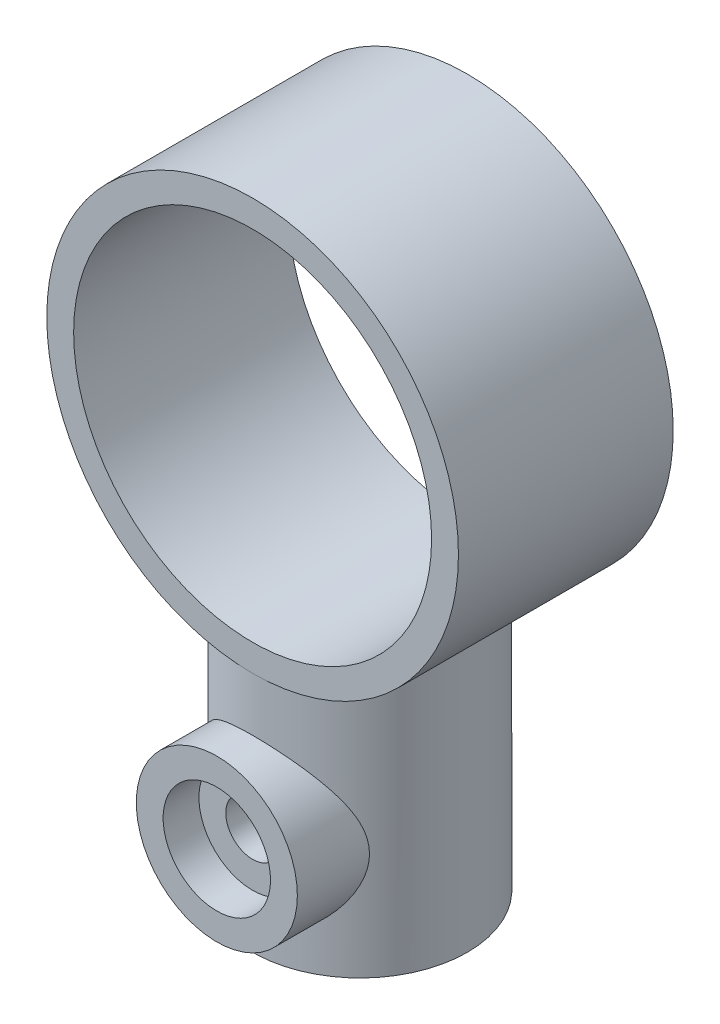
ISO-10303-21;
HEADER;
FILE_DESCRIPTION(('STEP AP214'),'2;1');
FILE_NAME('part.step','',(''),(''),'','','');
FILE_SCHEMA(('AUTOMOTIVE_DESIGN { 1 0 10303 214 1 1 1 1 }'));
ENDSEC;
DATA;
#1=APPLICATION_CONTEXT('core data for automotive mechanical design processes');
#2=APPLICATION_PROTOCOL_DEFINITION('international standard','automotive_design',2000,#1);
#3=PRODUCT_CONTEXT('',#1,'mechanical');
#4=PRODUCT('Part','Part','',(#3));
#5=PRODUCT_RELATED_PRODUCT_CATEGORY('part','',(#4));
#6=PRODUCT_DEFINITION_FORMATION('','',#4);
#7=PRODUCT_DEFINITION_CONTEXT('part definition',#1,'design');
#8=PRODUCT_DEFINITION('design','',#6,#7);
#9=PRODUCT_DEFINITION_SHAPE('','',#8);
#10=(LENGTH_UNIT() NAMED_UNIT(*) SI_UNIT(.MILLI.,.METRE.));
#11=(NAMED_UNIT(*) PLANE_ANGLE_UNIT() SI_UNIT($,.RADIAN.));
#12=(NAMED_UNIT(*) SI_UNIT($,.STERADIAN.) SOLID_ANGLE_UNIT());
#13=UNCERTAINTY_MEASURE_WITH_UNIT(LENGTH_MEASURE(1.E-05),#10,'distance_accuracy_value','');
#14=(GEOMETRIC_REPRESENTATION_CONTEXT(3) GLOBAL_UNCERTAINTY_ASSIGNED_CONTEXT((#13)) GLOBAL_UNIT_ASSIGNED_CONTEXT((#10,
#11,#12)) REPRESENTATION_CONTEXT('',''));
#15=CARTESIAN_POINT('',(0.,0.,0.));
#16=DIRECTION('',(0.,0.,1.));
#17=DIRECTION('',(1.,0.,0.));
#18=AXIS2_PLACEMENT_3D('',#15,#16,#17);
#19=CARTESIAN_POINT('',(0.,-19.,2.));
#20=DIRECTION('',(0.,0.,1.));
#21=DIRECTION('',(1.,0.,0.));
#22=AXIS2_PLACEMENT_3D('',#19,#20,#21);
#23=CYLINDRICAL_SURFACE('',#22,1.5);
#24=CARTESIAN_POINT('',(0.,-19.,6.));
#25=DIRECTION('',(0.,0.,1.));
#26=DIRECTION('',(1.,0.,0.));
#27=AXIS2_PLACEMENT_3D('',#24,#25,#26);
#28=CIRCLE('',#27,1.5);
#29=CARTESIAN_POINT('',(1.5,-19.,6.));
#30=VERTEX_POINT('',#29);
#31=EDGE_CURVE('E110',#30,#30,#28,.T.);
#32=ORIENTED_EDGE('',*,*,#31,.T.);
#33=EDGE_LOOP('',(#32));
#34=FACE_BOUND('',#33,.T.);
#35=CARTESIAN_POINT('',(0.,-19.,3.70809924354776));
#36=DIRECTION('',(0.,0.,-1.));
#37=DIRECTION('',(0.,1.,0.));
#38=AXIS2_PLACEMENT_3D('',#35,#36,#37);
#39=CIRCLE('',#38,1.5);
#40=CARTESIAN_POINT('',(-1.50000000000004,-18.9999999999999,3.70809924354776));
#41=VERTEX_POINT('',#40);
#42=CARTESIAN_POINT('',(1.49999999999977,-19.,3.70809924354776));
#43=VERTEX_POINT('',#42);
#44=EDGE_CURVE('E96',#41,#43,#39,.F.);
#45=ORIENTED_EDGE('',*,*,#44,.F.);
#46=EDGE_CURVE('E101',#43,#41,#39,.F.);
#47=ORIENTED_EDGE('',*,*,#46,.F.);
#48=EDGE_LOOP('',(#45,#47));
#49=FACE_BOUND('',#48,.T.);
#50=ADVANCED_FACE('F41',(#34,#49),#23,.F.);
#51=CARTESIAN_POINT('',(0.,-7.,3.70809924354776));
#52=DIRECTION('',(0.,0.,1.));
#53=DIRECTION('',(1.,0.,0.));
#54=AXIS2_PLACEMENT_3D('',#51,#52,#53);
#55=PLANE('',#54);
#56=ORIENTED_EDGE('',*,*,#46,.T.);
#57=DIRECTION('',(0.,-1.,0.));
#58=VECTOR('',#57,1.);
#59=CARTESIAN_POINT('',(-1.49999999999987,-6.99999999999999,3.70809924354776));
#60=LINE('',#59,#58);
#61=CARTESIAN_POINT('',(-1.49999999999991,-11.4017542509914,3.70809924354776));
#62=VERTEX_POINT('',#61);
#63=EDGE_CURVE('E83',#62,#41,#60,.T.);
#64=ORIENTED_EDGE('',*,*,#63,.F.);
#65=CARTESIAN_POINT('',(0.,0.,3.70809924354776));
#66=DIRECTION('',(0.,0.,1.));
#67=DIRECTION('',(1.,0.,0.));
#68=AXIS2_PLACEMENT_3D('',#65,#66,#67);
#69=CIRCLE('',#68,11.5);
#70=CARTESIAN_POINT('',(1.5000000000001,-11.4017542509914,3.70809924354776));
#71=VERTEX_POINT('',#70);
#72=EDGE_CURVE('E63',#62,#71,#69,.T.);
#73=ORIENTED_EDGE('',*,*,#72,.T.);
#74=DIRECTION('',(0.,-1.,0.));
#75=VECTOR('',#74,1.);
#76=CARTESIAN_POINT('',(1.50000000000013,-7.00000000000001,3.70809924354776));
#77=LINE('',#76,#75);
#78=EDGE_CURVE('E56',#71,#43,#77,.T.);
#79=ORIENTED_EDGE('',*,*,#78,.T.);
#80=EDGE_LOOP('',(#56,#64,#73,#79));
#81=FACE_BOUND('',#80,.T.);
#82=ADVANCED_FACE('F104',(#81),#55,.F.);
#83=CARTESIAN_POINT('',(0.,0.,6.));
#84=DIRECTION('',(0.,0.,1.));
#85=DIRECTION('',(1.,0.,0.));
#86=AXIS2_PLACEMENT_3D('',#83,#84,#85);
#87=PLANE('',#86);
#88=CARTESIAN_POINT('',(0.,0.,6.));
#89=DIRECTION('',(0.,0.,1.));
#90=DIRECTION('',(1.,0.,0.));
#91=AXIS2_PLACEMENT_3D('',#88,#89,#90);
#92=CIRCLE('',#91,11.5);
#93=CARTESIAN_POINT('',(0.,-11.5,6.));
#94=VERTEX_POINT('',#93);
#95=EDGE_CURVE('E51',#94,#94,#92,.T.);
#96=ORIENTED_EDGE('',*,*,#95,.T.);
#97=EDGE_LOOP('',(#96));
#98=FACE_BOUND('',#97,.T.);
#99=CARTESIAN_POINT('',(0.,0.,6.));
#100=DIRECTION('',(0.,0.,1.));
#101=DIRECTION('',(1.,0.,0.));
#102=AXIS2_PLACEMENT_3D('',#99,#100,#101);
#103=CIRCLE('',#102,10.);
#104=CARTESIAN_POINT('',(10.,0.,6.));
#105=VERTEX_POINT('',#104);
#106=EDGE_CURVE('E163',#105,#105,#103,.T.);
#107=ORIENTED_EDGE('',*,*,#106,.F.);
#108=EDGE_LOOP('',(#107));
#109=FACE_BOUND('',#108,.T.);
#110=ADVANCED_FACE('F180',(#98,#109),#87,.T.);
#111=CARTESIAN_POINT('',(0.,0.,-6.));
#112=DIRECTION('',(0.,0.,1.));
#113=DIRECTION('',(1.,0.,0.));
#114=AXIS2_PLACEMENT_3D('',#111,#112,#113);
#115=PLANE('',#114);
#116=CARTESIAN_POINT('',(0.,0.,-6.));
#117=DIRECTION('',(0.,0.,1.));
#118=DIRECTION('',(1.,0.,0.));
#119=AXIS2_PLACEMENT_3D('',#116,#117,#118);
#120=CIRCLE('',#119,11.5);
#121=CARTESIAN_POINT('',(0.,-11.5,-6.));
#122=VERTEX_POINT('',#121);
#123=EDGE_CURVE('E46',#122,#122,#120,.T.);
#124=ORIENTED_EDGE('',*,*,#123,.F.);
#125=EDGE_LOOP('',(#124));
#126=FACE_BOUND('',#125,.T.);
#127=CARTESIAN_POINT('',(0.,0.,-6.));
#128=DIRECTION('',(0.,0.,1.));
#129=DIRECTION('',(1.,0.,0.));
#130=AXIS2_PLACEMENT_3D('',#127,#128,#129);
#131=CIRCLE('',#130,10.);
#132=CARTESIAN_POINT('',(10.,0.,-6.));
#133=VERTEX_POINT('',#132);
#134=EDGE_CURVE('E152',#133,#133,#131,.T.);
#135=ORIENTED_EDGE('',*,*,#134,.T.);
#136=EDGE_LOOP('',(#135));
#137=FACE_BOUND('',#136,.T.);
#138=ADVANCED_FACE('F172',(#126,#137),#115,.F.);
#139=CARTESIAN_POINT('',(0.,0.,6.));
#140=DIRECTION('',(0.,0.,-1.));
#141=DIRECTION('',(-1.,0.,0.));
#142=AXIS2_PLACEMENT_3D('',#139,#140,#141);
#143=CYLINDRICAL_SURFACE('',#142,11.5);
#144=ORIENTED_EDGE('',*,*,#95,.F.);
#145=CARTESIAN_POINT('',(0.,-11.5,6.));
#146=CARTESIAN_POINT('',(0.156949578827933,-11.5000001355779,6.00000018262044));
#147=CARTESIAN_POINT('',(0.313897541694739,-11.496779962264,5.99383515190377));
#148=CARTESIAN_POINT('',(0.6266267232127,-11.4839818639018,5.969250324293));
#149=CARTESIAN_POINT('',(0.78240748044368,-11.4744015461444,5.95082591537107));
#150=CARTESIAN_POINT('',(1.09175175440838,-11.4491131770511,5.90191753135049));
#151=CARTESIAN_POINT('',(1.24531231034325,-11.4333976079975,5.87141876050534));
#152=CARTESIAN_POINT('',(1.54898348882044,-11.3962303126682,5.79871024455503));
#153=CARTESIAN_POINT('',(1.69909267420183,-11.374776242212,5.75649571329124));
#154=CARTESIAN_POINT('',(1.99416223199399,-11.3267626640489,5.66102891920833));
#155=CARTESIAN_POINT('',(2.13914255885142,-11.3002263208967,5.60782665445636));
#156=CARTESIAN_POINT('',(2.42383122801691,-11.242605583116,5.49078903598036));
#157=CARTESIAN_POINT('',(2.56353755744212,-11.2115194736562,5.42694967181545));
#158=CARTESIAN_POINT('',(2.97347192891126,-11.1124815994392,5.22033899187204));
#159=CARTESIAN_POINT('',(3.23482328089995,-11.0386979829443,5.06237435139018));
#160=CARTESIAN_POINT('',(3.74452958045316,-10.8767973262684,4.69923611516626));
#161=CARTESIAN_POINT('',(3.99097418237572,-10.7880643171826,4.49168348355608));
#162=CARTESIAN_POINT('',(4.44746391289357,-10.6080279075606,4.04018397814692));
#163=CARTESIAN_POINT('',(4.6574786381418,-10.5167224332789,3.79620701855532));
#164=CARTESIAN_POINT('',(4.95003726679143,-10.3807564849467,3.39525217625011));
#165=CARTESIAN_POINT('',(5.0470245263247,-10.3338194266377,3.24936331256475));
#166=CARTESIAN_POINT('',(5.22825678412554,-10.243318226809,2.94891015824408));
#167=CARTESIAN_POINT('',(5.31250719341773,-10.1997526568336,2.79434959010944));
#168=CARTESIAN_POINT('',(5.46751898205408,-10.1175068939615,2.47737077950324));
#169=CARTESIAN_POINT('',(5.53828138782099,-10.0788263293966,2.31495313612708));
#170=CARTESIAN_POINT('',(5.66549605291689,-10.007870040671,1.98334549078617));
#171=CARTESIAN_POINT('',(5.72195711983356,-9.97559037714009,1.81415973172985));
#172=CARTESIAN_POINT('',(5.81683662761796,-9.92054619063598,1.48073913098547));
#173=CARTESIAN_POINT('',(5.85614780407474,-9.8973202433967,1.3168349660179));
#174=CARTESIAN_POINT('',(5.92092061333041,-9.85870819120579,0.985481152489067));
#175=CARTESIAN_POINT('',(5.94638992234954,-9.84331774125878,0.818033522652497));
#176=CARTESIAN_POINT('',(5.98307546018686,-9.82106263754181,0.481141485903813));
#177=CARTESIAN_POINT('',(5.99430220671722,-9.81419169245379,0.311698645834845));
#178=CARTESIAN_POINT('',(6.00233545828585,-9.80928110826301,-0.0276480579803441));
#179=CARTESIAN_POINT('',(5.99914357072096,-9.81124048475133,-0.197551868226959));
#180=CARTESIAN_POINT('',(5.97979128876463,-9.82304398186212,-0.513523609621449));
#181=CARTESIAN_POINT('',(5.96541862727505,-9.83180084202554,-0.659746262263788));
#182=CARTESIAN_POINT('',(5.92608183096432,-9.85556101429158,-0.950290027245844));
#183=CARTESIAN_POINT('',(5.90111441248928,-9.87056626294257,-1.09461053574011));
#184=CARTESIAN_POINT('',(5.84088654816266,-9.90632463124338,-1.38034672465066));
#185=CARTESIAN_POINT('',(5.80562691028421,-9.92707729969527,-1.52176263215529));
#186=CARTESIAN_POINT('',(5.72519555337451,-9.97367980424175,-1.80090697735693));
#187=CARTESIAN_POINT('',(5.68001991596391,-9.99953165490475,-1.93863393312992));
#188=CARTESIAN_POINT('',(5.52798396598323,-10.0848968911938,-2.35127008986333));
#189=CARTESIAN_POINT('',(5.40595529204071,-10.1513811071149,-2.61932137568859));
#190=CARTESIAN_POINT('',(5.12582570187856,-10.2956624209485,-3.13233832170076));
#191=CARTESIAN_POINT('',(4.96770863914086,-10.3734645770196,-3.37729357882386));
#192=CARTESIAN_POINT('',(4.59418299191631,-10.5447319025564,-3.87335238223689));
#193=CARTESIAN_POINT('',(4.37385657367147,-10.6388667848999,-4.12053410943194));
#194=CARTESIAN_POINT('',(3.8945238655214,-10.8235162312259,-4.5762402813956));
#195=CARTESIAN_POINT('',(3.63549598915194,-10.9140287388105,-4.78474300580679));
#196=CARTESIAN_POINT('',(3.2143211161667,-11.0427084943076,-5.06942258731698));
#197=CARTESIAN_POINT('',(3.06415302608544,-11.0854180973587,-5.16160643824063));
#198=CARTESIAN_POINT('',(2.75534105655058,-11.1661770963876,-5.33284393580427));
#199=CARTESIAN_POINT('',(2.59670081324246,-11.2042284688993,-5.41190315646262));
#200=CARTESIAN_POINT('',(2.27203832366371,-11.274547726851,-5.55602186298455));
#201=CARTESIAN_POINT('',(2.10601941978374,-11.3068181982645,-5.62108761118107));
#202=CARTESIAN_POINT('',(1.76778722899716,-11.3646092392143,-5.73644830342684));
#203=CARTESIAN_POINT('',(1.59557472936085,-11.3901306632039,-5.78674511736463));
#204=CARTESIAN_POINT('',(1.26171558673617,-11.4317037739775,-5.86813103172292));
#205=CARTESIAN_POINT('',(1.10046276945584,-11.4483886224873,-5.90051563500229));
#206=CARTESIAN_POINT('',(0.775301200908844,-11.4749948435218,-5.9519739570192));
#207=CARTESIAN_POINT('',(0.611392714773712,-11.4849168870103,-5.9710489962542));
#208=CARTESIAN_POINT('',(0.282358074725133,-11.4977115427036,-5.99562178270494));
#209=CARTESIAN_POINT('',(0.117232478147314,-11.5005872021086,-6.00112539887258));
#210=CARTESIAN_POINT('',(-0.212876139333233,-11.4992139337846,-5.99849344051178));
#211=CARTESIAN_POINT('',(-0.377859167245579,-11.494965378924,-5.99035857979601));
#212=CARTESIAN_POINT('',(-0.692077607348148,-11.4801392838329,-5.96185612461983));
#213=CARTESIAN_POINT('',(-0.841443338858839,-11.4701395533605,-5.94260475543453));
#214=CARTESIAN_POINT('',(-1.1378856895511,-11.4445338372521,-5.89303027605832));
#215=CARTESIAN_POINT('',(-1.28496157460343,-11.4289260907783,-5.8627036883562));
#216=CARTESIAN_POINT('',(-1.57576547001364,-11.3924726565118,-5.791318826621));
#217=CARTESIAN_POINT('',(-1.71949451694579,-11.3716286147179,-5.7502639248081));
#218=CARTESIAN_POINT('',(-2.00284565139837,-11.3251593447799,-5.65781144649547));
#219=CARTESIAN_POINT('',(-2.1424661144892,-11.2995322541789,-5.6064098405095));
#220=CARTESIAN_POINT('',(-2.42036025169921,-11.2433297744297,-5.49226711627424));
#221=CARTESIAN_POINT('',(-2.55850470284527,-11.212643127812,-5.42926609647112));
#222=CARTESIAN_POINT('',(-2.82894302130084,-11.1474867251274,-5.29339248396464));
#223=CARTESIAN_POINT('',(-2.96123488974975,-11.1130156903428,-5.22051655263843));
#224=CARTESIAN_POINT('',(-3.3483703143814,-11.0050011672394,-4.98788532913089));
#225=CARTESIAN_POINT('',(-3.59362293177143,-10.9268248816615,-4.81406476637323));
#226=CARTESIAN_POINT('',(-4.07845441766789,-10.7558845893354,-4.41308062583474));
#227=CARTESIAN_POINT('',(-4.31476155891889,-10.6624498887889,-4.18224068751647));
#228=CARTESIAN_POINT('',(-4.63865684293523,-10.5236283447289,-3.80920784754676));
#229=CARTESIAN_POINT('',(-4.74159614201426,-10.4775407642408,-3.68029020728233));
#230=CARTESIAN_POINT('',(-4.93679704899914,-10.3869914671592,-3.41398249926734));
#231=CARTESIAN_POINT('',(-5.02905693172337,-10.3425300140459,-3.2765910681174));
#232=CARTESIAN_POINT('',(-5.2075334781137,-10.2538835713497,-2.98538298472546));
#233=CARTESIAN_POINT('',(-5.29304089939074,-10.2098799999887,-2.83107557841413));
#234=CARTESIAN_POINT('',(-5.45053097521659,-10.126679772442,-2.51454537611282));
#235=CARTESIAN_POINT('',(-5.52252016002734,-10.0874807984915,-2.35232644990204));
#236=CARTESIAN_POINT('',(-5.65216403762056,-10.0154153379937,-2.02105131937275));
#237=CARTESIAN_POINT('',(-5.70983122240028,-9.98254333857718,-1.85200122409345));
#238=CARTESIAN_POINT('',(-5.81010867727679,-9.9245153269321,-1.5082048281158));
#239=CARTESIAN_POINT('',(-5.85272151536941,-9.89935799881859,-1.33345950447928));
#240=CARTESIAN_POINT('',(-5.91879845654428,-9.8599773571974,-0.997125596417495));
#241=CARTESIAN_POINT('',(-5.94372747316176,-9.84492546066,-0.835921212389537));
#242=CARTESIAN_POINT('',(-5.98038742493029,-9.82269981291726,-0.511477725647174));
#243=CARTESIAN_POINT('',(-5.99211929476964,-9.81552550378242,-0.348238767859585));
#244=CARTESIAN_POINT('',(-6.00219018121771,-9.8093704244503,-0.0212746956513013));
#245=CARTESIAN_POINT('',(-6.00053582448525,-9.81038560016566,0.142450138120795));
#246=CARTESIAN_POINT('',(-5.98387835527532,-9.82055469279135,0.468955429442394));
#247=CARTESIAN_POINT('',(-5.96887599193873,-9.82970815295021,0.63173593947489));
#248=CARTESIAN_POINT('',(-5.92819127728147,-9.85429043436735,0.936742751821818));
#249=CARTESIAN_POINT('',(-5.90389851592604,-9.86889848594337,1.07922324730548));
#250=CARTESIAN_POINT('',(-5.8452817746423,-9.90372810988931,1.36142472318204));
#251=CARTESIAN_POINT('',(-5.81095451103383,-9.92395151971452,1.5011447842494));
#252=CARTESIAN_POINT('',(-5.69344223441867,-9.9921474078394,1.91488554677635));
#253=CARTESIAN_POINT('',(-5.59570137647601,-10.0476618132275,2.18367293189669));
#254=CARTESIAN_POINT('',(-5.35717564237041,-10.1769405832222,2.71886242225505));
#255=CARTESIAN_POINT('',(-5.21397923406328,-10.2516663146062,2.98394079537057));
#256=CARTESIAN_POINT('',(-4.89110956605737,-10.4095819630624,3.48808983239893));
#257=CARTESIAN_POINT('',(-4.71141672357178,-10.4927764121656,3.72714642766466));
#258=CARTESIAN_POINT('',(-4.29183181980609,-10.6718711921826,4.2065242224796));
#259=CARTESIAN_POINT('',(-4.04707182811816,-10.7679568339543,4.4425706468183));
#260=CARTESIAN_POINT('',(-3.65148746580848,-10.9057916851509,4.76399275734891));
#261=CARTESIAN_POINT('',(-3.51475503645127,-10.9507237321279,4.86576586077563));
#262=CARTESIAN_POINT('',(-3.23243661986418,-11.0373504171677,5.05771159354309));
#263=CARTESIAN_POINT('',(-3.08685463531819,-11.0790464997227,5.14788941081377));
#264=CARTESIAN_POINT('',(-2.78486276212116,-11.158825320879,5.31743165196371));
#265=CARTESIAN_POINT('',(-2.62830336717781,-11.196827869194,5.39656770964361));
#266=CARTESIAN_POINT('',(-2.30786598455693,-11.2672374830238,5.54117575722826));
#267=CARTESIAN_POINT('',(-2.14399164949471,-11.2996473027075,5.60665447609682));
#268=CARTESIAN_POINT('',(-1.81040554038446,-11.3578623353638,5.72307380861668));
#269=CARTESIAN_POINT('',(-1.64070671649361,-11.3836812442014,5.77404459543316));
#270=CARTESIAN_POINT('',(-1.29664056140096,-11.4279822417378,5.86090237441121));
#271=CARTESIAN_POINT('',(-1.12227597512963,-11.4464685472303,5.89679803659391));
#272=CARTESIAN_POINT('',(-0.79028551012749,-11.4738827208415,5.94982642127283));
#273=CARTESIAN_POINT('',(-0.632992460182356,-11.483654127812,5.96861998891456));
#274=CARTESIAN_POINT('',(-0.31713240879539,-11.4967127694845,5.99370682209347));
#275=CARTESIAN_POINT('',(-0.158565379695124,-11.4999998630263,5.99999981549947));
#276=CARTESIAN_POINT('',(0.,-11.5,6.));
#277=B_SPLINE_CURVE_WITH_KNOTS('',3,(#145,#146,#147,#148,#149,#150,#151,#152,#153,#154,#155,
#156,#157,#158,#159,#160,#161,#162,#163,#164,#165,#166,#167,#168,#169,#170,#171,#172,#173,#174,
#175,#176,#177,#178,#179,#180,#181,#182,#183,#184,#185,#186,#187,#188,#189,#190,#191,#192,#193,
#194,#195,#196,#197,#198,#199,#200,#201,#202,#203,#204,#205,#206,#207,#208,#209,#210,#211,#212,
#213,#214,#215,#216,#217,#218,#219,#220,#221,#222,#223,#224,#225,#226,#227,#228,#229,#230,#231,
#232,#233,#234,#235,#236,#237,#238,#239,#240,#241,#242,#243,#244,#245,#246,#247,#248,#249,#250,
#251,#252,#253,#254,#255,#256,#257,#258,#259,#260,#261,#262,#263,#264,#265,#266,#267,#268,#269,
#270,#271,#272,#273,#274,#275,#276),.UNSPECIFIED.,.T.,.F.,(4,2,2,2,2,2,2,2,2,2,2,2,2,2,2,2,2,2,
2,2,2,2,2,2,2,2,2,2,2,2,2,2,2,2,2,2,2,2,2,2,2,2,2,2,2,2,2,2,2,2,2,2,2,2,2,2,2,2,2,2,2,2,2,2,2,
4),(0.,0.470692988347527,0.941563153500217,1.41301211091961,1.88465395034882,2.35419515677509,
2.82391379370479,3.76237773296836,4.76106646584416,5.76058470750014,6.30410876981105,
6.8474012727456,7.39065241517701,7.93356817434236,8.4432575664312,8.95266401326091,
9.46169405906647,9.97066735933802,10.4117092732762,10.8528879801556,11.2940320623631,
11.7353507807,12.6372965018234,13.5396465616096,14.5680573329443,15.597043875982,
16.140352845317,16.6834304782373,17.2262645659939,17.7690298960917,18.2643078023531,
18.7595365630343,19.2545511248155,19.749539779258,20.2018125668466,20.6542274859734,
21.1065003686736,21.5589497293685,22.0231534673376,22.4875145420254,23.4157482798121,
24.4409922351983,24.9544170464423,25.4679246823015,26.0126762775516,26.557164038545,
27.1011752028526,27.6450935239605,28.1358290947884,28.6265299070667,29.1169878198374,
29.6074182079819,30.0427373760832,30.4781991573565,31.3485636603898,32.2762679094131,
33.2044712553565,34.2592761503955,34.7875907669549,35.3156681778426,35.8534199346152,
36.3909061122234,36.92726613486,37.4633172617339,37.9388456973503,38.4143844848669),.UNSPECIFIED.);
#278=EDGE_CURVE('E154',#94,#122,#277,.T.);
#279=ORIENTED_EDGE('',*,*,#278,.T.);
#280=ORIENTED_EDGE('',*,*,#123,.T.);
#281=EDGE_CURVE('E159',#122,#94,#277,.T.);
#282=ORIENTED_EDGE('',*,*,#281,.T.);
#283=EDGE_LOOP('',(#144,#279,#280,#282));
#284=FACE_BOUND('',#283,.T.);
#285=ADVANCED_FACE('F43',(#284),#143,.T.);
#286=CARTESIAN_POINT('',(0.,0.,6.));
#287=DIRECTION('',(0.,0.,-1.));
#288=DIRECTION('',(-1.,0.,0.));
#289=AXIS2_PLACEMENT_3D('',#286,#287,#288);
#290=CYLINDRICAL_SURFACE('',#289,10.);
#291=ORIENTED_EDGE('',*,*,#106,.T.);
#292=EDGE_LOOP('',(#291));
#293=FACE_BOUND('',#292,.T.);
#294=ORIENTED_EDGE('',*,*,#134,.F.);
#295=EDGE_LOOP('',(#294));
#296=FACE_BOUND('',#295,.T.);
#297=ADVANCED_FACE('F150',(#293,#296),#290,.F.);
#298=CARTESIAN_POINT('',(0.,-7.,0.));
#299=DIRECTION('',(0.,-1.,0.));
#300=DIRECTION('',(1.,0.,0.));
#301=AXIS2_PLACEMENT_3D('',#298,#299,#300);
#302=CYLINDRICAL_SURFACE('',#301,3.99999999999993);
#303=CARTESIAN_POINT('',(1.5,-25.,3.70809924354776));
#304=VERTEX_POINT('',#303);
#305=EDGE_CURVE('E91',#43,#304,#77,.T.);
#306=ORIENTED_EDGE('',*,*,#305,.F.);
#307=ORIENTED_EDGE('',*,*,#78,.F.);
#308=CARTESIAN_POINT('',(3.99999999999986,-10.781929326424,0.));
#309=CARTESIAN_POINT('',(4.00000314657652,-10.7819266948872,-0.217255336232914));
#310=CARTESIAN_POINT('',(3.98224047792889,-10.7885674998856,-0.434488763758288));
#311=CARTESIAN_POINT('',(3.91192630301894,-10.8142594176625,-0.862481103339597));
#312=CARTESIAN_POINT('',(3.85937154330999,-10.8333116910484,-1.07323940797085));
#313=CARTESIAN_POINT('',(3.72157378861011,-10.8814129934875,-1.48200382376832));
#314=CARTESIAN_POINT('',(3.6363995247052,-10.9104409900308,-1.68003573245359));
#315=CARTESIAN_POINT('',(3.43601854263587,-10.9751913442759,-2.05906879865697));
#316=CARTESIAN_POINT('',(3.32080431721443,-11.0109153747487,-2.2400656835589));
#317=CARTESIAN_POINT('',(3.05835039537032,-11.0867408076852,-2.58761009149744));
#318=CARTESIAN_POINT('',(2.9100429040825,-11.1269581781588,-2.75332615882137));
#319=CARTESIAN_POINT('',(2.58788673420046,-11.2062630333278,-3.05810823348963));
#320=CARTESIAN_POINT('',(2.41403354000832,-11.2453503167978,-3.19716951915368));
#321=CARTESIAN_POINT('',(2.03956351041542,-11.3193455391787,-3.44854433058932));
#322=CARTESIAN_POINT('',(1.83832180830089,-11.3541013537127,-3.55997575292531));
#323=CARTESIAN_POINT('',(1.41853124269149,-11.4141420626472,-3.74706935634629));
#324=CARTESIAN_POINT('',(1.19998750897693,-11.4394297515533,-3.82274209329461));
#325=CARTESIAN_POINT('',(0.760522326117555,-11.4768629954855,-3.93331855030355));
#326=CARTESIAN_POINT('',(0.539999668884433,-11.4894671957487,-3.96964898787937));
#327=CARTESIAN_POINT('',(0.0956518560104309,-11.5017473691412,-4.0050577250022));
#328=CARTESIAN_POINT('',(-0.128172356803093,-11.5014269643494,-4.00414646141529));
#329=CARTESIAN_POINT('',(-0.562628738311855,-11.4881984836479,-3.96597785288426));
#330=CARTESIAN_POINT('',(-0.773416363456932,-11.4758279465457,-3.930272591008));
#331=CARTESIAN_POINT('',(-1.18579631370684,-11.4405741640333,-3.82611095336748));
#332=CARTESIAN_POINT('',(-1.38738800209992,-11.4176901919009,-3.7576523135711));
#333=CARTESIAN_POINT('',(-1.77891248704159,-11.3633227238448,-3.58908505835547));
#334=CARTESIAN_POINT('',(-1.96864770310442,-11.3317257016856,-3.4885556579473));
#335=CARTESIAN_POINT('',(-2.32899682093034,-11.2631907969005,-3.25905514608549));
#336=CARTESIAN_POINT('',(-2.49960506659063,-11.2262513418015,-3.13007565484153));
#337=CARTESIAN_POINT('',(-2.82606513386257,-11.1486745512438,-2.83962735433131));
#338=CARTESIAN_POINT('',(-2.98072147863608,-11.1079447015802,-2.67683757838325));
#339=CARTESIAN_POINT('',(-3.26094797642742,-11.0289376993801,-2.32731693730578));
#340=CARTESIAN_POINT('',(-3.38651277882249,-10.9906609989707,-2.1405816778313));
#341=CARTESIAN_POINT('',(-3.60684990992326,-10.920360971299,-1.74437541164528));
#342=CARTESIAN_POINT('',(-3.7010718200857,-10.8884530012696,-1.53457624721657));
#343=CARTESIAN_POINT('',(-3.8524271261761,-10.8358341813979,-1.10069484305685));
#344=CARTESIAN_POINT('',(-3.90957773937398,-10.8151181343644,-0.876619286987419));
#345=CARTESIAN_POINT('',(-3.98263925841823,-10.7884212419073,-0.432210719646963));
#346=CARTESIAN_POINT('',(-4.00041969811956,-10.7817730993558,-0.212225215469678));
#347=CARTESIAN_POINT('',(-3.99956545239841,-10.7820910624059,0.227639507886412));
#348=CARTESIAN_POINT('',(-3.98093815848701,-10.789054404599,0.447518739575677));
#349=CARTESIAN_POINT('',(-3.90948277571084,-10.8151411210005,0.872074491886128));
#350=CARTESIAN_POINT('',(-3.8580010540821,-10.8337852906148,1.07701030192532));
#351=CARTESIAN_POINT('',(-3.7239397943008,-10.8805918133589,1.4752774913194));
#352=CARTESIAN_POINT('',(-3.64135444260578,-10.9087559457527,1.66860669346018));
#353=CARTESIAN_POINT('',(-3.44426879415293,-10.9726048973001,2.04541993178731));
#354=CARTESIAN_POINT('',(-3.32878445230759,-11.0085116691766,2.2283506225589));
#355=CARTESIAN_POINT('',(-3.07027059544534,-11.0833894368424,2.57290905730878));
#356=CARTESIAN_POINT('',(-2.92723227768871,-11.1223614095187,2.73452996552629));
#357=CARTESIAN_POINT('',(-2.60865742371181,-11.2014821658468,3.04076690570169));
#358=CARTESIAN_POINT('',(-2.43179808769057,-11.2415834741986,3.18402336891874));
#359=CARTESIAN_POINT('',(-2.05556021379345,-11.3164220998505,3.43893786266677));
#360=CARTESIAN_POINT('',(-1.85618224045722,-11.3511595515703,3.55059668510105));
#361=CARTESIAN_POINT('',(-1.44132125531167,-11.4112320794752,3.73819420931193));
#362=CARTESIAN_POINT('',(-1.22593857393044,-11.436620625482,3.81433673175178));
#363=CARTESIAN_POINT('',(-0.784357241241908,-11.4753568277292,3.92896429388479));
#364=CARTESIAN_POINT('',(-0.558162920245526,-11.488709262854,3.96746427989474));
#365=CARTESIAN_POINT('',(-0.113762111596045,-11.501476627674,4.00427643177558));
#366=CARTESIAN_POINT('',(0.104265596272577,-11.5015658253351,4.00453280420546));
#367=CARTESIAN_POINT('',(0.537113760489189,-11.4894896642182,3.96971528088925));
#368=CARTESIAN_POINT('',(0.751934515174897,-11.4773254526561,3.93464469260193));
#369=CARTESIAN_POINT('',(1.1682689825417,-11.4423785548636,3.83148907745086));
#370=CARTESIAN_POINT('',(1.36995572166124,-11.4197972370693,3.76402918727062));
#371=CARTESIAN_POINT('',(1.75920776274612,-11.3663462696473,3.59860185717365));
#372=CARTESIAN_POINT('',(1.94677043880624,-11.3354750836387,3.50062876163337));
#373=CARTESIAN_POINT('',(2.31041493756695,-11.2671005300579,3.27258612737591));
#374=CARTESIAN_POINT('',(2.48576658696086,-11.2293859263638,3.14141652896516));
#375=CARTESIAN_POINT('',(2.8125947319369,-11.1520208071119,2.85252769438948));
#376=CARTESIAN_POINT('',(2.96406324330576,-11.1123696499352,2.6947996159213));
#377=CARTESIAN_POINT('',(3.24557817237721,-11.0335192560423,2.34905234319778));
#378=CARTESIAN_POINT('',(3.37440059236079,-10.9944153308317,2.16001130869306));
#379=CARTESIAN_POINT('',(3.59839984489605,-10.9231587605909,1.76172989505965));
#380=CARTESIAN_POINT('',(3.69358164349432,-10.8910050898327,1.55249250313871));
#381=CARTESIAN_POINT('',(3.8458069995994,-10.838183085146,1.12288270167076));
#382=CARTESIAN_POINT('',(3.90342389063485,-10.8173429457616,0.90273569256634));
#383=CARTESIAN_POINT('',(3.98051046462658,-10.7892203865282,0.455048945321354));
#384=CARTESIAN_POINT('',(3.99999670486609,-10.7819320822016,0.227512459529251));
#385=CARTESIAN_POINT('',(3.99999999999986,-10.781929326424,0.));
#386=B_SPLINE_CURVE_WITH_KNOTS('',3,(#308,#309,#310,#311,#312,#313,#314,#315,#316,#317,#318,
#319,#320,#321,#322,#323,#324,#325,#326,#327,#328,#329,#330,#331,#332,#333,#334,#335,#336,#337,
#338,#339,#340,#341,#342,#343,#344,#345,#346,#347,#348,#349,#350,#351,#352,#353,#354,#355,#356,
#357,#358,#359,#360,#361,#362,#363,#364,#365,#366,#367,#368,#369,#370,#371,#372,#373,#374,#375,
#376,#377,#378,#379,#380,#381,#382,#383,#384,#385),.UNSPECIFIED.,.T.,.F.,(4,2,2,2,2,2,2,2,2,2,2,
2,2,2,2,2,2,2,2,2,2,2,2,2,2,2,2,2,2,2,2,2,2,2,2,2,2,2,4),(0.,0.650921909801569,1.301904696625,
1.95152330718617,2.60130441915738,3.27625918225249,3.95133339788453,4.64578028679665,
5.34002204868048,6.00814477227088,6.67608025791707,7.31552343393114,7.95501081696127,
8.60325980697967,9.25169999011812,9.93319342368778,10.6148121006922,11.3078365129701,
12.0005388284013,12.6595705401675,13.3184684689778,13.9519613616294,14.5855727184921,
15.2405921689976,15.8958212283479,16.5858602431942,17.2758819626803,17.9618935348493,
18.6476326090358,19.298497953293,19.9493023664602,20.5880220121539,21.2268601150802,
21.8905428059991,22.5544469000047,23.2473366731027,23.9401241186769,24.6220737318841,
25.3037271597275),.UNSPECIFIED.);
#387=EDGE_CURVE('E94',#71,#62,#386,.T.);
#388=ORIENTED_EDGE('',*,*,#387,.T.);
#389=ORIENTED_EDGE('',*,*,#63,.T.);
#390=CARTESIAN_POINT('',(-1.5,-25.,3.70809924354776));
#391=VERTEX_POINT('',#390);
#392=EDGE_CURVE('E87',#41,#391,#60,.T.);
#393=ORIENTED_EDGE('',*,*,#392,.T.);
#394=CARTESIAN_POINT('',(-1.74574066942157E-13,-25.,0.));
#395=DIRECTION('',(0.,-1.,0.));
#396=DIRECTION('',(1.,0.,0.));
#397=AXIS2_PLACEMENT_3D('',#394,#395,#396);
#398=CIRCLE('',#397,3.99999999999993);
#399=EDGE_CURVE('E304',#391,#304,#398,.T.);
#400=ORIENTED_EDGE('',*,*,#399,.T.);
#401=EDGE_LOOP('',(#306,#307,#388,#389,#393,#400));
#402=FACE_BOUND('',#401,.T.);
#403=ADVANCED_FACE('F90',(#402),#302,.F.);
#404=CARTESIAN_POINT('',(0.,-7.,0.));
#405=DIRECTION('',(0.,-1.,0.));
#406=DIRECTION('',(1.,0.,0.));
#407=AXIS2_PLACEMENT_3D('',#404,#405,#406);
#408=CYLINDRICAL_SURFACE('',#407,6.);
#409=CARTESIAN_POINT('',(4.5,-19.,3.96862696659674));
#410=CARTESIAN_POINT('',(4.50000507834795,-18.8949418488794,3.96861686602141));
#411=CARTESIAN_POINT('',(4.49631419586517,-18.7899195297317,3.9728168514459));
#412=CARTESIAN_POINT('',(4.48167225616228,-18.5809864703694,3.98932854522559));
#413=CARTESIAN_POINT('',(4.47071877665906,-18.4770761127793,4.00164295996579));
#414=CARTESIAN_POINT('',(4.44180872189387,-18.2711836297107,4.03370728475386));
#415=CARTESIAN_POINT('',(4.42383673572161,-18.1692062688658,4.0534735539058));
#416=CARTESIAN_POINT('',(4.38129405910782,-17.9680882523386,4.09941990164114));
#417=CARTESIAN_POINT('',(4.35671931259617,-17.8689493819012,4.12560392177298));
#418=CARTESIAN_POINT('',(4.2745464375733,-17.5794046616541,4.21122557626126));
#419=CARTESIAN_POINT('',(4.20803426948237,-17.3937238166576,4.2782871478847));
#420=CARTESIAN_POINT('',(4.05390989402713,-17.0369234945698,4.42460194939479));
#421=CARTESIAN_POINT('',(3.96630023685819,-16.865802260941,4.50385370535392));
#422=CARTESIAN_POINT('',(3.75120672461474,-16.5036814358669,4.68531341730841));
#423=CARTESIAN_POINT('',(3.61921460613341,-16.3160250828106,4.78885287141302));
#424=CARTESIAN_POINT('',(3.32798047453307,-15.9623946729377,4.99564919290693));
#425=CARTESIAN_POINT('',(3.16869833241079,-15.7964531900511,5.09890541333791));
#426=CARTESIAN_POINT('',(2.89258319383621,-15.5500278679837,5.25807588714212));
#427=CARTESIAN_POINT('',(2.78403025278295,-15.4617866905745,5.31649921498468));
#428=CARTESIAN_POINT('',(2.55764383078975,-15.2948357833496,5.42903557769024));
#429=CARTESIAN_POINT('',(2.43980827260277,-15.2161281970001,5.48314764230636));
#430=CARTESIAN_POINT('',(2.19555612221116,-15.0693791398114,5.58542936763));
#431=CARTESIAN_POINT('',(2.06915634837481,-15.0013175852969,5.63361018010819));
#432=CARTESIAN_POINT('',(1.80839242601433,-14.8768220679997,5.72264868834265));
#433=CARTESIAN_POINT('',(1.67403253937859,-14.8203819542008,5.76351025654372));
#434=CARTESIAN_POINT('',(1.34369921738147,-14.7004313389689,5.85098111190473));
#435=CARTESIAN_POINT('',(1.14436283139104,-14.6429432828994,5.89347882975045));
#436=CARTESIAN_POINT('',(0.736633167118957,-14.5558150938569,5.95818156512857));
#437=CARTESIAN_POINT('',(0.528247922690005,-14.5261507664387,5.98040421262311));
#438=CARTESIAN_POINT('',(0.107601910306231,-14.4963387137746,6.00273790900922));
#439=CARTESIAN_POINT('',(-0.104667502038748,-14.4962676849033,6.00279150279406));
#440=CARTESIAN_POINT('',(-0.525950245750392,-14.5258527620655,5.98062709423097));
#441=CARTESIAN_POINT('',(-0.734962811689901,-14.5555157523132,5.95840393422351));
#442=CARTESIAN_POINT('',(-1.1366671291912,-14.6412434187138,5.894741109369));
#443=CARTESIAN_POINT('',(-1.32967268311153,-14.6963690509536,5.85398567140417));
#444=CARTESIAN_POINT('',(-1.70304157676307,-14.8299868547386,5.75646842129022));
#445=CARTESIAN_POINT('',(-1.88340214926541,-14.9084841213365,5.69970311910817));
#446=CARTESIAN_POINT('',(-2.24765072773045,-15.0955888678264,5.56683136038156));
#447=CARTESIAN_POINT('',(-2.42980614387423,-15.2065362960667,5.48929621311769));
#448=CARTESIAN_POINT('',(-2.77370176192021,-15.4502011056958,5.32382107964188));
#449=CARTESIAN_POINT('',(-2.9354243570541,-15.5829370386549,5.23587224475466));
#450=CARTESIAN_POINT('',(-3.26724612468181,-15.8956700493885,5.03681297456608));
#451=CARTESIAN_POINT('',(-3.43273478808483,-16.0798276340312,4.92454967628694));
#452=CARTESIAN_POINT('',(-3.7320262687465,-16.4735037469118,4.70177874821722));
#453=CARTESIAN_POINT('',(-3.86581399076325,-16.683034285684,4.59127197811539));
#454=CARTESIAN_POINT('',(-4.07619618880002,-17.0829456210872,4.40458278221533));
#455=CARTESIAN_POINT('',(-4.15886599457748,-17.2689611706744,4.32592800158741));
#456=CARTESIAN_POINT('',(-4.299581924703,-17.6561958095648,4.1861022298521));
#457=CARTESIAN_POINT('',(-4.35768369642175,-17.8573793107592,4.12489183040217));
#458=CARTESIAN_POINT('',(-4.43707152670479,-18.231060934876,4.03920154203046));
#459=CARTESIAN_POINT('',(-4.46337197039467,-18.4013415947896,4.00984626605542));
#460=CARTESIAN_POINT('',(-4.4961529329497,-18.7460660505289,3.97306757390269));
#461=CARTESIAN_POINT('',(-4.5026588096003,-18.9205042312478,3.96561609832594));
#462=CARTESIAN_POINT('',(-4.49535767990839,-19.268438264135,3.9738863572465));
#463=CARTESIAN_POINT('',(-4.48154319688052,-19.4419337458683,3.98961662125101));
#464=CARTESIAN_POINT('',(-4.43467740096359,-19.7832236406719,4.04163546634424));
#465=CARTESIAN_POINT('',(-4.40159325331274,-19.9510078040983,4.07795913497766));
#466=CARTESIAN_POINT('',(-4.30241066255206,-20.3390388580603,4.18283837891074));
#467=CARTESIAN_POINT('',(-4.22859010341975,-20.5554161651888,4.25836937509181));
#468=CARTESIAN_POINT('',(-4.09668298226637,-20.8654438394661,4.38416713744612));
#469=CARTESIAN_POINT('',(-4.04911000925131,-20.9664833861314,4.42824776609358));
#470=CARTESIAN_POINT('',(-3.94721295720349,-21.1637489343204,4.51931162288282));
#471=CARTESIAN_POINT('',(-3.89288948793118,-21.2599753695043,4.56629458866908));
#472=CARTESIAN_POINT('',(-3.71615208503641,-21.5479802978199,4.71319006454602));
#473=CARTESIAN_POINT('',(-3.58306413099202,-21.7318577243483,4.81595841514054));
#474=CARTESIAN_POINT('',(-3.29043603837122,-22.0780472133115,5.02045330209735));
#475=CARTESIAN_POINT('',(-3.13088304866243,-22.2403487294049,5.12217930670168));
#476=CARTESIAN_POINT('',(-2.85363567533699,-22.4822642002401,5.27933355837751));
#477=CARTESIAN_POINT('',(-2.74391171722391,-22.5694257365634,5.33733448882732));
#478=CARTESIAN_POINT('',(-2.51521929055212,-22.7341036187197,5.44883911627991));
#479=CARTESIAN_POINT('',(-2.39624873344224,-22.811617775131,5.50234179153681));
#480=CARTESIAN_POINT('',(-2.14976703494837,-22.9558619151249,5.60323071595807));
#481=CARTESIAN_POINT('',(-2.0222708370229,-23.0226101026115,5.65062726191324));
#482=CARTESIAN_POINT('',(-1.75941796478033,-23.1443250504998,5.73791214360097));
#483=CARTESIAN_POINT('',(-1.62406558315525,-23.1992981693023,5.77780453006821));
#484=CARTESIAN_POINT('',(-1.29236039433713,-23.3152591812484,5.86253509046218));
#485=CARTESIAN_POINT('',(-1.09277519250811,-23.3702557030909,5.90325172436765));
#486=CARTESIAN_POINT('',(-0.685068396776642,-23.4524010525127,5.96432057289535));
#487=CARTESIAN_POINT('',(-0.476954608596302,-23.4795747777541,5.98469099424159));
#488=CARTESIAN_POINT('',(-0.05744953861628,-23.5045452304643,6.00340361255943));
#489=CARTESIAN_POINT('',(0.153948278458814,-23.5022729966562,6.00169409922427));
#490=CARTESIAN_POINT('',(0.573028832872338,-23.4683180817659,5.97626500489893));
#491=CARTESIAN_POINT('',(0.780710565484102,-23.4366275656964,5.9525395603943));
#492=CARTESIAN_POINT('',(1.1805653438649,-23.3470749807735,5.88610179466108));
#493=CARTESIAN_POINT('',(1.37301358555468,-23.2899993841215,5.8439606605958));
#494=CARTESIAN_POINT('',(1.7449841532986,-23.1526358750723,5.74388168045802));
#495=CARTESIAN_POINT('',(1.92450370414699,-23.0723429974141,5.68594045552011));
#496=CARTESIAN_POINT('',(2.28764305847085,-22.8811661683899,5.5505292444447));
#497=CARTESIAN_POINT('',(2.4694237039432,-22.7678472155168,5.47159056710834));
#498=CARTESIAN_POINT('',(2.81224444137565,-22.5194006687327,5.30356519640336));
#499=CARTESIAN_POINT('',(2.97326522407366,-22.384253030849,5.21446919850886));
#500=CARTESIAN_POINT('',(3.30337143548397,-22.0659839689441,5.01319054977127));
#501=CARTESIAN_POINT('',(3.46775082401069,-21.878661089558,4.89992751303398));
#502=CARTESIAN_POINT('',(3.76425752510146,-21.478395496317,4.67598263606579));
#503=CARTESIAN_POINT('',(3.89637302120337,-21.2654434384235,4.56530175491716));
#504=CARTESIAN_POINT('',(4.10087937073653,-20.863351097747,4.38148756734095));
#505=CARTESIAN_POINT('',(4.18000656903787,-20.6789979060429,4.30540715099529));
#506=CARTESIAN_POINT('',(4.31416116404688,-20.2957484143158,4.17097853448595));
#507=CARTESIAN_POINT('',(4.36925255772108,-20.0968923993726,4.11258337465181));
#508=CARTESIAN_POINT('',(4.43991376358635,-19.7476427827061,4.03596853197048));
#509=CARTESIAN_POINT('',(4.46233401591205,-19.6001227683933,4.01099047058807));
#510=CARTESIAN_POINT('',(4.49236863125038,-19.3017090349621,3.9773322850993));
#511=CARTESIAN_POINT('',(4.49999270971154,-19.1508175954789,3.96864146660904));
#512=CARTESIAN_POINT('',(4.5,-19.,3.96862696659674));
#513=B_SPLINE_CURVE_WITH_KNOTS('',3,(#409,#410,#411,#412,#413,#414,#415,#416,#417,#418,#419,
#420,#421,#422,#423,#424,#425,#426,#427,#428,#429,#430,#431,#432,#433,#434,#435,#436,#437,#438,
#439,#440,#441,#442,#443,#444,#445,#446,#447,#448,#449,#450,#451,#452,#453,#454,#455,#456,#457,
#458,#459,#460,#461,#462,#463,#464,#465,#466,#467,#468,#469,#470,#471,#472,#473,#474,#475,#476,
#477,#478,#479,#480,#481,#482,#483,#484,#485,#486,#487,#488,#489,#490,#491,#492,#493,#494,#495,
#496,#497,#498,#499,#500,#501,#502,#503,#504,#505,#506,#507,#508,#509,#510,#511,#512),
.UNSPECIFIED.,.T.,.F.,(4,2,2,2,2,2,2,2,2,2,2,2,2,2,2,2,2,2,2,2,2,2,2,2,2,2,2,2,2,2,2,2,2,2,2,2,
2,2,2,2,2,2,2,2,2,2,2,2,2,2,2,4),(0.,0.314967992529362,0.630041088741448,0.945809933215818,
1.26177319948834,1.88414018859977,2.50643198575638,3.25906029247442,4.01280496269483,
4.46706137040636,4.921419721134,5.37491031193945,5.82816025795598,6.46055479293374,
7.09239891072842,7.72588055644129,8.35950890384574,8.97143571145859,9.58349601786717,
10.2618283581139,10.940741281237,11.7532085507481,12.566061924045,13.218705318923,
13.8698624329972,14.3919632009841,14.9133948507529,15.4350184043935,15.9575333954877,
16.6756238806791,17.0355922774016,17.3955281824151,18.1405045759424,18.8858437866391,
19.3402547507058,19.7947686536145,20.2485057859157,20.7019972842675,21.3320515125033,
21.9615414328459,22.5925058597018,23.2236383798888,23.8364490074278,24.4493907880505,
25.1317662013588,25.8147717990099,26.6328920440152,27.4513114729265,28.0930130158956,
28.7329953998515,29.1854489890177,29.6376053879207),.UNSPECIFIED.);
#514=CARTESIAN_POINT('',(4.5,-19.,3.96862696659674));
#515=VERTEX_POINT('',#514);
#516=EDGE_CURVE('E11',#515,#515,#513,.T.);
#517=ORIENTED_EDGE('',*,*,#516,.F.);
#518=EDGE_LOOP('',(#517));
#519=FACE_BOUND('',#518,.T.);
#520=CARTESIAN_POINT('',(-1.74574066942157E-13,-25.,0.));
#521=DIRECTION('',(0.,-1.,0.));
#522=DIRECTION('',(1.,0.,0.));
#523=AXIS2_PLACEMENT_3D('',#520,#521,#522);
#524=CIRCLE('',#523,6.);
#525=CARTESIAN_POINT('',(5.99999999999983,-25.,0.));
#526=VERTEX_POINT('',#525);
#527=EDGE_CURVE('E118',#526,#526,#524,.T.);
#528=ORIENTED_EDGE('',*,*,#527,.F.);
#529=EDGE_LOOP('',(#528));
#530=FACE_BOUND('',#529,.T.);
#531=ORIENTED_EDGE('',*,*,#278,.F.);
#532=ORIENTED_EDGE('',*,*,#281,.F.);
#533=EDGE_LOOP('',(#531,#532));
#534=FACE_BOUND('',#533,.T.);
#535=ADVANCED_FACE('F130',(#519,#530,#534),#408,.T.);
#536=ORIENTED_EDGE('',*,*,#392,.F.);
#537=ORIENTED_EDGE('',*,*,#44,.T.);
#538=ORIENTED_EDGE('',*,*,#305,.T.);
#539=DIRECTION('',(-1.,0.,0.));
#540=VECTOR('',#539,1.);
#541=CARTESIAN_POINT('',(-1.77294687069391E-13,-25.,3.70809924354776));
#542=LINE('',#541,#540);
#543=EDGE_CURVE('E103',#304,#391,#542,.T.);
#544=ORIENTED_EDGE('',*,*,#543,.T.);
#545=EDGE_LOOP('',(#536,#537,#538,#544));
#546=FACE_BOUND('',#545,.T.);
#547=ADVANCED_FACE('F98',(#546),#55,.F.);
#548=CARTESIAN_POINT('',(-1.77294687069391E-13,-25.,0.));
#549=DIRECTION('',(0.,-1.,0.));
#550=DIRECTION('',(1.,0.,0.));
#551=AXIS2_PLACEMENT_3D('',#548,#549,#550);
#552=PLANE('',#551);
#553=ORIENTED_EDGE('',*,*,#527,.T.);
#554=EDGE_LOOP('',(#553));
#555=FACE_BOUND('',#554,.T.);
#556=ORIENTED_EDGE('',*,*,#399,.F.);
#557=ORIENTED_EDGE('',*,*,#543,.F.);
#558=EDGE_LOOP('',(#556,#557));
#559=FACE_BOUND('',#558,.T.);
#560=ADVANCED_FACE('F137',(#555,#559),#552,.T.);
#561=ORIENTED_EDGE('',*,*,#387,.F.);
#562=ORIENTED_EDGE('',*,*,#72,.F.);
#563=EDGE_LOOP('',(#561,#562));
#564=FACE_BOUND('',#563,.T.);
#565=ADVANCED_FACE('F136',(#564),#143,.T.);
#566=CARTESIAN_POINT('',(0.,-19.,2.));
#567=DIRECTION('',(0.,0.,1.));
#568=DIRECTION('',(1.,0.,0.));
#569=AXIS2_PLACEMENT_3D('',#566,#567,#568);
#570=CYLINDRICAL_SURFACE('',#569,4.5);
#571=ORIENTED_EDGE('',*,*,#516,.T.);
#572=EDGE_LOOP('',(#571));
#573=FACE_BOUND('',#572,.T.);
#574=CARTESIAN_POINT('',(0.,-19.,8.));
#575=DIRECTION('',(0.,0.,1.));
#576=DIRECTION('',(1.,0.,0.));
#577=AXIS2_PLACEMENT_3D('',#574,#575,#576);
#578=CIRCLE('',#577,4.5);
#579=CARTESIAN_POINT('',(4.5,-19.,8.));
#580=VERTEX_POINT('',#579);
#581=EDGE_CURVE('E114',#580,#580,#578,.T.);
#582=ORIENTED_EDGE('',*,*,#581,.F.);
#583=EDGE_LOOP('',(#582));
#584=FACE_BOUND('',#583,.T.);
#585=ADVANCED_FACE('F133',(#573,#584),#570,.T.);
#586=CARTESIAN_POINT('',(0.,-19.,8.));
#587=DIRECTION('',(0.,0.,1.));
#588=DIRECTION('',(1.,0.,0.));
#589=AXIS2_PLACEMENT_3D('',#586,#587,#588);
#590=PLANE('',#589);
#591=CARTESIAN_POINT('',(0.,-19.,8.));
#592=DIRECTION('',(0.,0.,1.));
#593=DIRECTION('',(1.,0.,0.));
#594=AXIS2_PLACEMENT_3D('',#591,#592,#593);
#595=CIRCLE('',#594,3.);
#596=CARTESIAN_POINT('',(3.,-19.,8.));
#597=VERTEX_POINT('',#596);
#598=EDGE_CURVE('E107',#597,#597,#595,.T.);
#599=ORIENTED_EDGE('',*,*,#598,.F.);
#600=EDGE_LOOP('',(#599));
#601=FACE_BOUND('',#600,.T.);
#602=ORIENTED_EDGE('',*,*,#581,.T.);
#603=EDGE_LOOP('',(#602));
#604=FACE_BOUND('',#603,.T.);
#605=ADVANCED_FACE('F139',(#601,#604),#590,.T.);
#606=CARTESIAN_POINT('',(0.,-19.,6.));
#607=DIRECTION('',(0.,0.,1.));
#608=DIRECTION('',(1.,0.,0.));
#609=AXIS2_PLACEMENT_3D('',#606,#607,#608);
#610=CYLINDRICAL_SURFACE('',#609,3.);
#611=CARTESIAN_POINT('',(0.,-19.,6.));
#612=DIRECTION('',(0.,0.,1.));
#613=DIRECTION('',(1.,0.,0.));
#614=AXIS2_PLACEMENT_3D('',#611,#612,#613);
#615=CIRCLE('',#614,3.);
#616=CARTESIAN_POINT('',(3.,-19.,6.));
#617=VERTEX_POINT('',#616);
#618=EDGE_CURVE('E115',#617,#617,#615,.T.);
#619=ORIENTED_EDGE('',*,*,#618,.F.);
#620=EDGE_LOOP('',(#619));
#621=FACE_BOUND('',#620,.T.);
#622=ORIENTED_EDGE('',*,*,#598,.T.);
#623=EDGE_LOOP('',(#622));
#624=FACE_BOUND('',#623,.T.);
#625=ADVANCED_FACE('F191',(#621,#624),#610,.F.);
#626=CARTESIAN_POINT('',(0.,-19.,6.));
#627=DIRECTION('',(0.,0.,1.));
#628=DIRECTION('',(1.,0.,0.));
#629=AXIS2_PLACEMENT_3D('',#626,#627,#628);
#630=PLANE('',#629);
#631=ORIENTED_EDGE('',*,*,#31,.F.);
#632=EDGE_LOOP('',(#631));
#633=FACE_BOUND('',#632,.T.);
#634=ORIENTED_EDGE('',*,*,#618,.T.);
#635=EDGE_LOOP('',(#634));
#636=FACE_BOUND('',#635,.T.);
#637=ADVANCED_FACE('F200',(#633,#636),#630,.T.);
#638=CLOSED_SHELL('',(#50,#82,#110,#138,#285,#297,#403,#535,#547,#560,#565,#585,#605,#625,#637));
#639=MANIFOLD_SOLID_BREP('B2',#638);
#640=ADVANCED_BREP_SHAPE_REPRESENTATION('',(#18,#639),#14);
#641=SHAPE_DEFINITION_REPRESENTATION(#9,#640);
ENDSEC;
END-ISO-10303-21;
